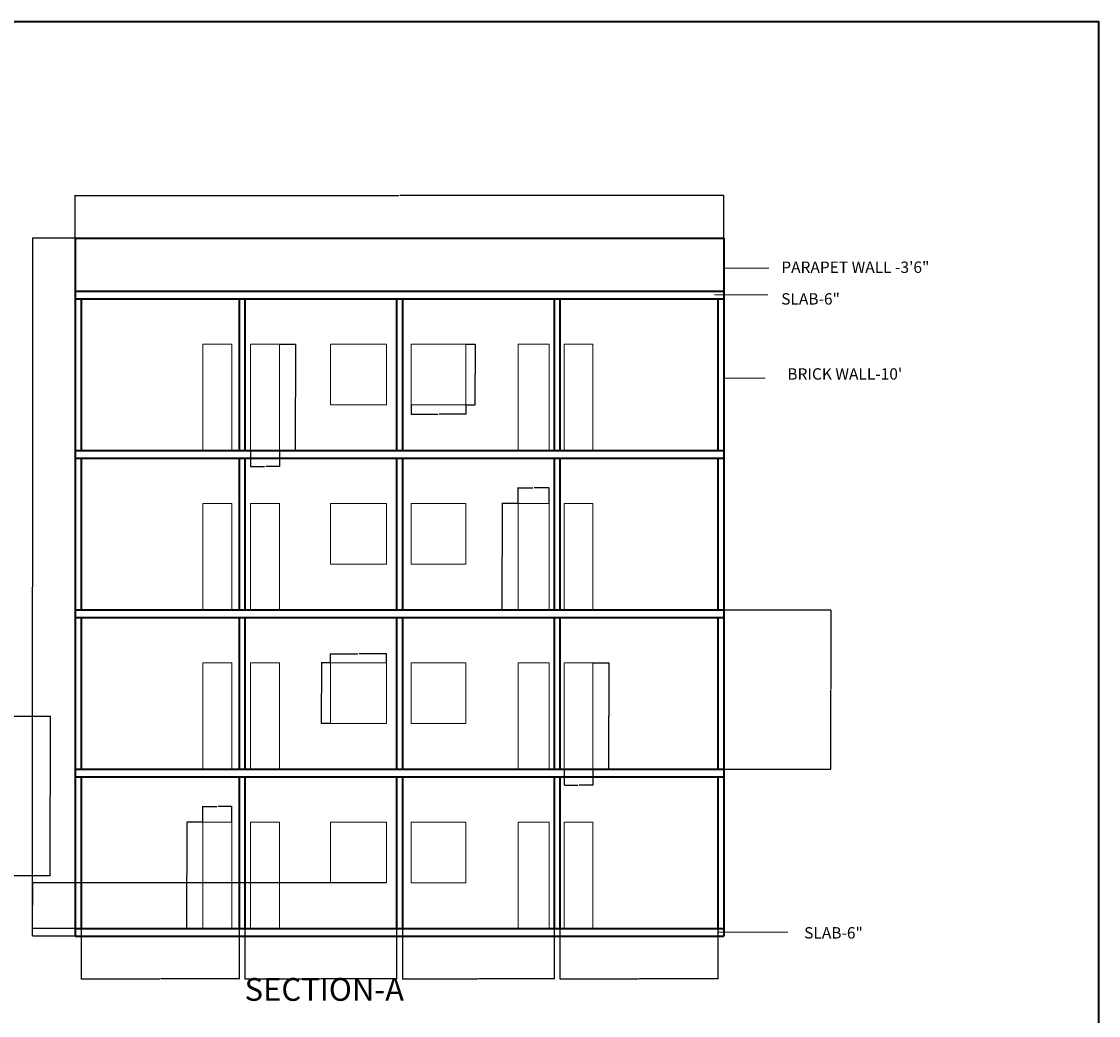
# Model space of a CAD drawing. Units: inches. Extents: x 1944 to 3454, y 1352 to 3055.
# Tile 17 of 17: x 2602 to 3454, y 2269 to 3055. Entities that reach past the tile are written whole.
import ezdxf

# ---------------------------------------------------------------- set-up
doc = ezdxf.new("R2010")
doc.units = ezdxf.units.IN
for name, color, linetype, lineweight in [('A-ANNO-DIMS', 2, 'Continuous', 18), ('A-ANNO-TEXT', 7, 'Continuous', 18), ('A-ANNO-TITL', 7, 'Continuous', 30), ('A-ANNO-TTLB', 7, 'Continuous', 35), ('A-SECT', 7, 'Continuous', 40), ('A-SECT-BYND', 8, 'Continuous', 18)]:
    doc.layers.add(name, color=color, linetype=linetype, lineweight=lineweight)
doc.styles.get("Standard").update_dxf_attribs({"font": 'arial.ttf'})
doc.dimstyles.get("Standard").update_dxf_attribs({"dimtxt": 0.18, "dimasz": 0.18, "dimexe": 0.18, "dimexo": 0.0625, "dimgap": 0.09, "dimtad": 0, "dimtih": 1, "dimtoh": 1, "dimdec": 4, "dimzin": 0, "dimdsep": 46, "dimtxsty": 'Standard', "dimcen": 0.09, "dimadec": 0, "dimazin": 0, "dimtfac": 1, "dimtdec": 4, "dimtofl": 0, "dimtmove": 0, "dimatfit": 3, "dimfxl": 1, "dimtolj": 1, "dimtzin": 0, "dimarcsym": 0})

# ---------------------------------------------------------------- blocks, each defined once
blk = doc.blocks.new('SECT-DOOR-22.85IN-01')
for p, q in [((0, 84), (0, 0)), ((0, 84), (22.85, 84)), ((22.85, 84), (22.85, 0))]:
    blk.add_line(p, q)
blk = doc.blocks.new('SECT-DOOR-23.10IN-01')
for p, q in [((0, 84), (0, 0)), ((0, 84), (23.1, 84)), ((23.1, 84), (23.1, 0))]:
    blk.add_line(p, q)
blk = doc.blocks.new('SECT-DOOR-24.49IN-01')
for p, q in [((0, 84), (0, 0)), ((0, 84), (24.49, 84)), ((24.49, 84), (24.49, 0))]:
    blk.add_line(p, q)
blk = doc.blocks.new('SECT-DOOR-22.62IN-01')
for p, q in [((0, 84), (0, 0)), ((0, 84), (22.62, 84)), ((22.62, 84), (22.62, 0))]:
    blk.add_line(p, q)
blk = doc.blocks.new('SECT-GLAZ-44.19IN-01')
for p, q in [((0, 48), (0, 0)), ((0, 48), (44.19, 48)), ((44.19, 48), (44.19, 0)), ((0, 0), (44.19, 0))]:
    blk.add_line(p, q)
blk = doc.blocks.new('SECT-GLAZ-43.38IN-01')
for p, q in [((0, 48), (0, 0)), ((0, 48), (43.38, 48)), ((43.38, 48), (43.38, 0)), ((0, 0), (43.38, 0))]:
    blk.add_line(p, q)
blk = doc.blocks.new('*D172')
at = {"layer": 'A-ANNO-DIMS', "color": 0, "lineweight": -2, "transparency": 16777216}
for p, q in [((2745.67, 2421.38), (2732.95, 2421.38)), ((2733.13, 2421.2), (2733.13, 2379.57)), ((2733.13, 2337.56), (2733.13, 2379.2)), ((2745.67, 2337.38), (2732.95, 2337.38))]:
    blk.add_line(p, q, dxfattribs=at)
at = {"layer": 'A-ANNO-DIMS', "color": 0, "transparency": 16777216}
for points in [[(2733.1, 2421.2), (2733.16, 2421.2), (2733.13, 2421.38)], [(2733.1, 2337.56), (2733.16, 2337.56), (2733.13, 2337.38)]]:
    blk.add_solid(points, dxfattribs=at)
at = {"layer": 'Defpoints', "color": 0, "transparency": 16777216}
for p in [(2733.13, 2421.38), (2745.73, 2421.38), (2745.73, 2337.38)]:
    blk.add_point(p, dxfattribs=at)
at = {"layer": 'A-ANNO-DIMS', "color": 0, "transparency": 16777216, "insert": (2733.13, 2379.38), "char_height": 0.18, "attachment_point": 5}
blk.add_mtext('\\A1;DOOR 84 TYP.', dxfattribs=at)
blk = doc.blocks.new('*D173')
at = {"layer": 'A-ANNO-DIMS', "color": 0, "lineweight": -2, "transparency": 16777216}
for p, q in [((2745.73, 2421.45), (2745.73, 2434.16)), ((2745.91, 2433.98), (2756.63, 2433.98)), ((2768.4, 2433.98), (2757.69, 2433.98)), ((2768.58, 2421.45), (2768.58, 2434.16))]:
    blk.add_line(p, q, dxfattribs=at)
at = {"layer": 'A-ANNO-DIMS', "color": 0, "transparency": 16777216}
for points in [[(2745.91, 2434.01), (2745.91, 2433.95), (2745.73, 2433.98)], [(2768.4, 2434.01), (2768.4, 2433.95), (2768.58, 2433.98)]]:
    blk.add_solid(points, dxfattribs=at)
at = {"layer": 'Defpoints', "color": 0, "transparency": 16777216}
for p in [(2768.58, 2433.98), (2745.73, 2421.38), (2768.58, 2421.38)]:
    blk.add_point(p, dxfattribs=at)
at = {"layer": 'A-ANNO-DIMS', "color": 0, "transparency": 16777216, "insert": (2757.16, 2433.98), "char_height": 0.18, "attachment_point": 5}
blk.add_mtext('\\A1;23 TYP.', dxfattribs=at)
blk = doc.blocks.new('*D174')
at = {"layer": 'A-ANNO-DIMS', "color": 0, "lineweight": -2, "transparency": 16777216}
for p, q in [((2806.45, 2799.38), (2819.17, 2799.38)), ((2818.99, 2799.2), (2818.99, 2757.57)), ((2818.99, 2715.56), (2818.99, 2757.2)), ((2806.45, 2715.38), (2819.17, 2715.38))]:
    blk.add_line(p, q, dxfattribs=at)
at = {"layer": 'A-ANNO-DIMS', "color": 0, "transparency": 16777216}
for points in [[(2818.96, 2799.2), (2819.02, 2799.2), (2818.99, 2799.38)], [(2818.96, 2715.56), (2819.02, 2715.56), (2818.99, 2715.38)]]:
    blk.add_solid(points, dxfattribs=at)
at = {"layer": 'Defpoints', "color": 0, "transparency": 16777216}
for p in [(2806.39, 2799.38), (2818.99, 2799.38), (2806.39, 2715.38)]:
    blk.add_point(p, dxfattribs=at)
at = {"layer": 'A-ANNO-DIMS', "color": 0, "transparency": 16777216, "insert": (2818.99, 2757.38), "char_height": 0.18, "attachment_point": 5}
blk.add_mtext('\\A1;DOOR 84 TYP.', dxfattribs=at)
blk = doc.blocks.new('*D175')
at = {"layer": 'A-ANNO-DIMS', "color": 0, "lineweight": -2, "transparency": 16777216}
for p, q in [((2783.29, 2715.32), (2783.29, 2702.6)), ((2806.39, 2715.32), (2806.39, 2702.6)), ((2783.47, 2702.78), (2794.31, 2702.78)), ((2806.21, 2702.78), (2795.37, 2702.78))]:
    blk.add_line(p, q, dxfattribs=at)
at = {"layer": 'A-ANNO-DIMS', "color": 0, "transparency": 16777216}
for points in [[(2783.47, 2702.81), (2783.47, 2702.75), (2783.29, 2702.78)], [(2806.21, 2702.81), (2806.21, 2702.75), (2806.39, 2702.78)]]:
    blk.add_solid(points, dxfattribs=at)
at = {"layer": 'Defpoints', "color": 0, "transparency": 16777216}
for p in [(2783.29, 2715.38), (2806.39, 2715.38), (2806.39, 2702.78)]:
    blk.add_point(p, dxfattribs=at)
at = {"layer": 'A-ANNO-DIMS', "color": 0, "transparency": 16777216, "insert": (2794.84, 2702.78), "char_height": 0.18, "attachment_point": 5}
blk.add_mtext('\\A1;23 TYP.', dxfattribs=at)
blk = doc.blocks.new('*D176')
at = {"layer": 'A-ANNO-DIMS', "color": 0, "lineweight": -2, "transparency": 16777216}
for p, q in [((2994.82, 2673.38), (2982.11, 2673.38)), ((2982.29, 2673.2), (2982.29, 2631.57)), ((2982.29, 2589.56), (2982.29, 2631.2)), ((2994.82, 2589.38), (2982.11, 2589.38))]:
    blk.add_line(p, q, dxfattribs=at)
at = {"layer": 'A-ANNO-DIMS', "color": 0, "transparency": 16777216}
for points in [[(2982.26, 2673.2), (2982.32, 2673.2), (2982.29, 2673.38)], [(2982.26, 2589.56), (2982.32, 2589.56), (2982.29, 2589.38)]]:
    blk.add_solid(points, dxfattribs=at)
at = {"layer": 'Defpoints', "color": 0, "transparency": 16777216}
for p in [(2982.29, 2673.38), (2994.89, 2673.38), (2994.89, 2589.38)]:
    blk.add_point(p, dxfattribs=at)
at = {"layer": 'A-ANNO-DIMS', "color": 0, "transparency": 16777216, "insert": (2982.29, 2631.38), "char_height": 0.18, "attachment_point": 5}
blk.add_mtext('\\A1;DOOR 84 TYP.', dxfattribs=at)
blk = doc.blocks.new('*D177')
at = {"layer": 'A-ANNO-DIMS', "color": 0, "lineweight": -2, "transparency": 16777216}
for p, q in [((2994.89, 2673.45), (2994.89, 2686.16)), ((2995.07, 2685.98), (3006.6, 2685.98)), ((3019.2, 2685.98), (3007.66, 2685.98)), ((3019.38, 2673.45), (3019.38, 2686.16))]:
    blk.add_line(p, q, dxfattribs=at)
at = {"layer": 'A-ANNO-DIMS', "color": 0, "transparency": 16777216}
for points in [[(2995.07, 2686.01), (2995.07, 2685.95), (2994.89, 2685.98)], [(3019.2, 2686.01), (3019.2, 2685.95), (3019.38, 2685.98)]]:
    blk.add_solid(points, dxfattribs=at)
at = {"layer": 'Defpoints', "color": 0, "transparency": 16777216}
for p in [(3019.38, 2685.98), (2994.89, 2673.38), (3019.38, 2673.38)]:
    blk.add_point(p, dxfattribs=at)
at = {"layer": 'A-ANNO-DIMS', "color": 0, "transparency": 16777216, "insert": (3007.13, 2685.98), "char_height": 0.18, "attachment_point": 5}
blk.add_mtext('\\A1;24 TYP.', dxfattribs=at)
blk = doc.blocks.new('*D178')
at = {"layer": 'A-ANNO-DIMS', "color": 0, "lineweight": -2, "transparency": 16777216}
for p, q in [((3054.1, 2547.38), (3066.81, 2547.38)), ((3066.63, 2547.2), (3066.63, 2505.57)), ((3066.63, 2463.56), (3066.63, 2505.2)), ((3054.1, 2463.38), (3066.81, 2463.38))]:
    blk.add_line(p, q, dxfattribs=at)
at = {"layer": 'A-ANNO-DIMS', "color": 0, "transparency": 16777216}
for points in [[(3066.6, 2547.2), (3066.66, 2547.2), (3066.63, 2547.38)], [(3066.6, 2463.56), (3066.66, 2463.56), (3066.63, 2463.38)]]:
    blk.add_solid(points, dxfattribs=at)
at = {"layer": 'Defpoints', "color": 0, "transparency": 16777216}
for p in [(3054.03, 2547.38), (3066.63, 2547.38), (3054.03, 2463.38)]:
    blk.add_point(p, dxfattribs=at)
at = {"layer": 'A-ANNO-DIMS', "color": 0, "transparency": 16777216, "insert": (3066.63, 2505.38), "char_height": 0.18, "attachment_point": 5}
blk.add_mtext('\\A1;DOOR 84 TYP.', dxfattribs=at)
blk = doc.blocks.new('*D179')
at = {"layer": 'A-ANNO-DIMS', "color": 0, "lineweight": -2, "transparency": 16777216}
for p, q in [((3031.42, 2463.32), (3031.42, 2450.6)), ((3054.03, 2463.32), (3054.03, 2450.6)), ((3031.6, 2450.78), (3042.2, 2450.78)), ((3053.85, 2450.78), (3043.26, 2450.78))]:
    blk.add_line(p, q, dxfattribs=at)
at = {"layer": 'A-ANNO-DIMS', "color": 0, "transparency": 16777216}
for points in [[(3031.6, 2450.81), (3031.6, 2450.75), (3031.42, 2450.78)], [(3053.85, 2450.81), (3053.85, 2450.75), (3054.03, 2450.78)]]:
    blk.add_solid(points, dxfattribs=at)
at = {"layer": 'Defpoints', "color": 0, "transparency": 16777216}
for p in [(3031.42, 2463.38), (3054.03, 2463.38), (3054.03, 2450.78)]:
    blk.add_point(p, dxfattribs=at)
at = {"layer": 'A-ANNO-DIMS', "color": 0, "transparency": 16777216, "insert": (3042.73, 2450.78), "char_height": 0.18, "attachment_point": 5}
blk.add_mtext('\\A1;23 TYP.', dxfattribs=at)
blk = doc.blocks.new('*D180')
at = {"layer": 'A-ANNO-DIMS', "color": 0, "lineweight": -2, "transparency": 16777216}
for p, q in [((2846.48, 2547.38), (2839.17, 2547.38)), ((2839.35, 2547.2), (2839.35, 2523.57)), ((2839.35, 2499.56), (2839.35, 2523.2)), ((2846.48, 2499.38), (2839.17, 2499.38))]:
    blk.add_line(p, q, dxfattribs=at)
at = {"layer": 'A-ANNO-DIMS', "color": 0, "transparency": 16777216}
for points in [[(2839.32, 2547.2), (2839.38, 2547.2), (2839.35, 2547.38)], [(2839.32, 2499.56), (2839.38, 2499.56), (2839.35, 2499.38)]]:
    blk.add_solid(points, dxfattribs=at)
at = {"layer": 'Defpoints', "color": 0, "transparency": 16777216}
for p in [(2839.35, 2547.38), (2846.55, 2547.38), (2846.55, 2499.38)]:
    blk.add_point(p, dxfattribs=at)
at = {"layer": 'A-ANNO-DIMS', "color": 0, "transparency": 16777216, "insert": (2839.35, 2523.38), "char_height": 0.18, "attachment_point": 5}
blk.add_mtext('\\A1;GLAZING 48 TYP.', dxfattribs=at)
blk = doc.blocks.new('*D181')
at = {"layer": 'A-ANNO-DIMS', "color": 0, "lineweight": -2, "transparency": 16777216}
for p, q in [((2846.55, 2547.45), (2846.55, 2554.76)), ((2846.73, 2554.58), (2868.11, 2554.58)), ((2890.56, 2554.58), (2869.17, 2554.58)), ((2890.74, 2547.45), (2890.74, 2554.76))]:
    blk.add_line(p, q, dxfattribs=at)
at = {"layer": 'A-ANNO-DIMS', "color": 0, "transparency": 16777216}
for points in [[(2846.73, 2554.61), (2846.73, 2554.55), (2846.55, 2554.58)], [(2890.56, 2554.61), (2890.56, 2554.55), (2890.74, 2554.58)]]:
    blk.add_solid(points, dxfattribs=at)
at = {"layer": 'Defpoints', "color": 0, "transparency": 16777216}
for p in [(2890.74, 2554.58), (2846.55, 2547.38), (2890.74, 2547.38)]:
    blk.add_point(p, dxfattribs=at)
at = {"layer": 'A-ANNO-DIMS', "color": 0, "transparency": 16777216, "insert": (2868.64, 2554.58), "char_height": 0.18, "attachment_point": 5}
blk.add_mtext('\\A1;44 TYP.', dxfattribs=at)
blk = doc.blocks.new('*D182')
at = {"layer": 'A-ANNO-DIMS', "color": 0, "lineweight": -2, "transparency": 16777216}
for p, q in [((2953.72, 2799.38), (2961.03, 2799.38)), ((2960.85, 2799.2), (2960.85, 2775.57)), ((2960.85, 2751.56), (2960.85, 2775.2)), ((2953.72, 2751.38), (2961.03, 2751.38))]:
    blk.add_line(p, q, dxfattribs=at)
at = {"layer": 'A-ANNO-DIMS', "color": 0, "transparency": 16777216}
for points in [[(2960.82, 2799.2), (2960.88, 2799.2), (2960.85, 2799.38)], [(2960.82, 2751.56), (2960.88, 2751.56), (2960.85, 2751.38)]]:
    blk.add_solid(points, dxfattribs=at)
at = {"layer": 'Defpoints', "color": 0, "transparency": 16777216}
for p in [(2953.65, 2799.38), (2960.85, 2799.38), (2953.65, 2751.38)]:
    blk.add_point(p, dxfattribs=at)
at = {"layer": 'A-ANNO-DIMS', "color": 0, "transparency": 16777216, "insert": (2960.85, 2775.38), "char_height": 0.18, "attachment_point": 5}
blk.add_mtext('\\A1;GLAZING 48 TYP.', dxfattribs=at)
blk = doc.blocks.new('*D183')
at = {"layer": 'A-ANNO-DIMS', "color": 0, "lineweight": -2, "transparency": 16777216}
for p, q in [((2910.28, 2751.32), (2910.28, 2744)), ((2953.65, 2751.32), (2953.65, 2744)), ((2910.46, 2744.18), (2931.43, 2744.18)), ((2953.47, 2744.18), (2932.5, 2744.18))]:
    blk.add_line(p, q, dxfattribs=at)
at = {"layer": 'A-ANNO-DIMS', "color": 0, "transparency": 16777216}
for points in [[(2910.46, 2744.21), (2910.46, 2744.15), (2910.28, 2744.18)], [(2953.47, 2744.21), (2953.47, 2744.15), (2953.65, 2744.18)]]:
    blk.add_solid(points, dxfattribs=at)
at = {"layer": 'Defpoints', "color": 0, "transparency": 16777216}
for p in [(2910.28, 2751.38), (2953.65, 2751.38), (2953.65, 2744.18)]:
    blk.add_point(p, dxfattribs=at)
at = {"layer": 'A-ANNO-DIMS', "color": 0, "transparency": 16777216, "insert": (2931.96, 2744.18), "char_height": 0.18, "attachment_point": 5}
blk.add_mtext('\\A1;43 TYP.', dxfattribs=at)
blk = doc.blocks.new('*D201')
at = {"layer": 'A-ANNO-DIMS', "color": 0, "lineweight": -2, "transparency": 16777216}
for p, q in [((2593.88, 2505.38), (2625.2, 2505.38)), ((2625.02, 2505.2), (2625.02, 2442.57)), ((2625.02, 2379.56), (2625.02, 2442.2)), ((2593.88, 2379.38), (2625.2, 2379.38))]:
    blk.add_line(p, q, dxfattribs=at)
at = {"layer": 'A-ANNO-DIMS', "color": 0, "transparency": 16777216}
for points in [[(2624.99, 2505.2), (2625.05, 2505.2), (2625.02, 2505.38)], [(2624.99, 2379.56), (2625.05, 2379.56), (2625.02, 2379.38)]]:
    blk.add_solid(points, dxfattribs=at)
at = {"layer": 'Defpoints', "color": 0, "transparency": 16777216}
for p in [(2593.82, 2505.38), (2625.02, 2505.38), (2593.82, 2379.38)]:
    blk.add_point(p, dxfattribs=at)
at = {"layer": 'A-ANNO-DIMS', "color": 0, "transparency": 16777216, "insert": (2625.02, 2442.38), "char_height": 0.18, "attachment_point": 5}
blk.add_mtext('\\A1;126', dxfattribs=at)
blk = doc.blocks.new('*D209')
at = {"layer": 'A-ANNO-DIMS', "color": 0, "lineweight": -2, "transparency": 16777216}
for p, q in [((2644.88, 2883.45), (2644.88, 2917.33)), ((2645.06, 2917.15), (2900.73, 2917.15)), ((3157.2, 2917.15), (2901.52, 2917.15)), ((3157.38, 2883.45), (3157.38, 2917.33))]:
    blk.add_line(p, q, dxfattribs=at)
at = {"layer": 'A-ANNO-DIMS', "color": 0, "transparency": 16777216}
for points in [[(2645.06, 2917.18), (2645.06, 2917.12), (2644.88, 2917.15)], [(3157.2, 2917.18), (3157.2, 2917.12), (3157.38, 2917.15)]]:
    blk.add_solid(points, dxfattribs=at)
at = {"layer": 'Defpoints', "color": 0, "transparency": 16777216}
for p in [(3157.38, 2917.15), (2644.88, 2883.38), (3157.38, 2883.38)]:
    blk.add_point(p, dxfattribs=at)
at = {"layer": 'A-ANNO-DIMS', "color": 0, "transparency": 16777216, "insert": (2901.13, 2917.15), "char_height": 0.18, "attachment_point": 5}
blk.add_mtext('\\A1;512.5', dxfattribs=at)
blk = doc.blocks.new('*D210')
at = {"layer": 'A-ANNO-DIMS', "color": 0, "lineweight": -2, "transparency": 16777216}
for p, q in [((2644.81, 2883.38), (2610.93, 2883.38)), ((2611.11, 2883.2), (2611.11, 2607.57)), ((2611.11, 2331.56), (2611.11, 2607.2)), ((2644.81, 2331.38), (2610.93, 2331.38))]:
    blk.add_line(p, q, dxfattribs=at)
at = {"layer": 'A-ANNO-DIMS', "color": 0, "transparency": 16777216}
for points in [[(2611.08, 2883.2), (2611.14, 2883.2), (2611.11, 2883.38)], [(2611.08, 2331.56), (2611.14, 2331.56), (2611.11, 2331.38)]]:
    blk.add_solid(points, dxfattribs=at)
at = {"layer": 'Defpoints', "color": 0, "transparency": 16777216}
for p in [(2611.11, 2883.38), (2644.88, 2883.38), (2644.88, 2331.38)]:
    blk.add_point(p, dxfattribs=at)
at = {"layer": 'A-ANNO-DIMS', "color": 0, "transparency": 16777216, "insert": (2611.11, 2607.38), "char_height": 0.18, "attachment_point": 5}
blk.add_mtext('\\A1;552', dxfattribs=at)
blk = doc.blocks.new('*D211')
at = {"layer": 'A-ANNO-DIMS', "color": 0, "lineweight": -2, "transparency": 16777216}
for p, q in [((3157.44, 2589.38), (3242.15, 2589.38)), ((3241.97, 2589.2), (3241.97, 2526.57)), ((3241.97, 2463.56), (3241.97, 2526.2)), ((3157.44, 2463.38), (3242.15, 2463.38))]:
    blk.add_line(p, q, dxfattribs=at)
at = {"layer": 'A-ANNO-DIMS', "color": 0, "transparency": 16777216}
for points in [[(3241.94, 2589.2), (3242, 2589.2), (3241.97, 2589.38)], [(3241.94, 2463.56), (3242, 2463.56), (3241.97, 2463.38)]]:
    blk.add_solid(points, dxfattribs=at)
at = {"layer": 'Defpoints', "color": 0, "transparency": 16777216}
for p in [(3157.38, 2589.38), (3241.97, 2589.38), (3157.38, 2463.38)]:
    blk.add_point(p, dxfattribs=at)
at = {"layer": 'A-ANNO-DIMS', "color": 0, "transparency": 16777216, "insert": (3241.97, 2526.38), "char_height": 0.18, "attachment_point": 5}
blk.add_mtext('\\A1;126', dxfattribs=at)
blk = doc.blocks.new('*D212')
at = {"layer": 'A-ANNO-DIMS', "color": 0, "lineweight": -2, "transparency": 16777216}
for p, q in [((2649.38, 2337.32), (2649.38, 2297.43)), ((2774.38, 2337.32), (2774.38, 2297.43)), ((2649.56, 2297.61), (2711.59, 2297.61)), ((2774.2, 2297.61), (2712.16, 2297.61))]:
    blk.add_line(p, q, dxfattribs=at)
at = {"layer": 'A-ANNO-DIMS', "color": 0, "transparency": 16777216}
for points in [[(2649.56, 2297.64), (2649.56, 2297.58), (2649.38, 2297.61)], [(2774.2, 2297.64), (2774.2, 2297.58), (2774.38, 2297.61)]]:
    blk.add_solid(points, dxfattribs=at)
at = {"layer": 'Defpoints', "color": 0, "transparency": 16777216}
for p in [(2649.38, 2337.38), (2774.38, 2337.38), (2774.38, 2297.61)]:
    blk.add_point(p, dxfattribs=at)
at = {"layer": 'A-ANNO-DIMS', "color": 0, "transparency": 16777216, "insert": (2711.88, 2297.61), "char_height": 0.18, "attachment_point": 5}
blk.add_mtext('\\A1;125', dxfattribs=at)
blk = doc.blocks.new('*D213')
at = {"layer": 'A-ANNO-DIMS', "color": 0, "lineweight": -2, "transparency": 16777216}
for p, q in [((2778.88, 2337.32), (2778.88, 2297.43)), ((2898.88, 2337.32), (2898.88, 2297.43)), ((2779.06, 2297.61), (2838.6, 2297.61)), ((2898.7, 2297.61), (2839.16, 2297.61))]:
    blk.add_line(p, q, dxfattribs=at)
at = {"layer": 'A-ANNO-DIMS', "color": 0, "transparency": 16777216}
for points in [[(2779.06, 2297.64), (2779.06, 2297.58), (2778.88, 2297.61)], [(2898.7, 2297.64), (2898.7, 2297.58), (2898.88, 2297.61)]]:
    blk.add_solid(points, dxfattribs=at)
at = {"layer": 'Defpoints', "color": 0, "transparency": 16777216}
for p in [(2778.88, 2337.38), (2898.88, 2337.38), (2898.88, 2297.61)]:
    blk.add_point(p, dxfattribs=at)
at = {"layer": 'A-ANNO-DIMS', "color": 0, "transparency": 16777216, "insert": (2838.88, 2297.61), "char_height": 0.18, "attachment_point": 5}
blk.add_mtext('\\A1;120', dxfattribs=at)
blk = doc.blocks.new('*D214')
at = {"layer": 'A-ANNO-DIMS', "color": 0, "lineweight": -2, "transparency": 16777216}
for p, q in [((2903.38, 2337.32), (2903.38, 2297.43)), ((3023.38, 2337.32), (3023.38, 2297.43)), ((2903.56, 2297.61), (2963.1, 2297.61)), ((3023.2, 2297.61), (2963.66, 2297.61))]:
    blk.add_line(p, q, dxfattribs=at)
at = {"layer": 'A-ANNO-DIMS', "color": 0, "transparency": 16777216}
for points in [[(2903.56, 2297.64), (2903.56, 2297.58), (2903.38, 2297.61)], [(3023.2, 2297.64), (3023.2, 2297.58), (3023.38, 2297.61)]]:
    blk.add_solid(points, dxfattribs=at)
at = {"layer": 'Defpoints', "color": 0, "transparency": 16777216}
for p in [(2903.38, 2337.38), (3023.38, 2337.38), (3023.38, 2297.61)]:
    blk.add_point(p, dxfattribs=at)
at = {"layer": 'A-ANNO-DIMS', "color": 0, "transparency": 16777216, "insert": (2963.38, 2297.61), "char_height": 0.18, "attachment_point": 5}
blk.add_mtext('\\A1;120', dxfattribs=at)
blk = doc.blocks.new('*D215')
at = {"layer": 'A-ANNO-DIMS', "color": 0, "lineweight": -2, "transparency": 16777216}
for p, q in [((3027.88, 2337.32), (3027.88, 2297.43)), ((3152.88, 2337.32), (3152.88, 2297.43)), ((3028.06, 2297.61), (3090.09, 2297.61)), ((3152.7, 2297.61), (3090.66, 2297.61))]:
    blk.add_line(p, q, dxfattribs=at)
at = {"layer": 'A-ANNO-DIMS', "color": 0, "transparency": 16777216}
for points in [[(3028.06, 2297.64), (3028.06, 2297.58), (3027.88, 2297.61)], [(3152.7, 2297.64), (3152.7, 2297.58), (3152.88, 2297.61)]]:
    blk.add_solid(points, dxfattribs=at)
at = {"layer": 'Defpoints', "color": 0, "transparency": 16777216}
for p in [(3027.88, 2337.38), (3152.88, 2337.38), (3152.88, 2297.61)]:
    blk.add_point(p, dxfattribs=at)
at = {"layer": 'A-ANNO-DIMS', "color": 0, "transparency": 16777216, "insert": (3090.38, 2297.61), "char_height": 0.18, "attachment_point": 5}
blk.add_mtext('\\A1;125', dxfattribs=at)
blk = doc.blocks.new('*D216')
at = {"layer": 'A-ANNO-DIMS', "color": 0, "lineweight": -2, "transparency": 16777216}
for p, q in [((2890.68, 2373.38), (2610.93, 2373.38)), ((2611.11, 2373.2), (2611.11, 2355.57)), ((2611.11, 2337.56), (2611.11, 2355.2)), ((2898.81, 2337.38), (2610.93, 2337.38))]:
    blk.add_line(p, q, dxfattribs=at)
at = {"layer": 'A-ANNO-DIMS', "color": 0, "transparency": 16777216}
for points in [[(2611.08, 2373.2), (2611.14, 2373.2), (2611.11, 2373.38)], [(2611.08, 2337.56), (2611.14, 2337.56), (2611.11, 2337.38)]]:
    blk.add_solid(points, dxfattribs=at)
at = {"layer": 'Defpoints', "color": 0, "transparency": 16777216}
for p in [(2611.11, 2373.38), (2890.74, 2373.38), (2898.88, 2337.38)]:
    blk.add_point(p, dxfattribs=at)
at = {"layer": 'A-ANNO-DIMS', "color": 0, "transparency": 16777216, "insert": (2611.11, 2355.38), "char_height": 0.18, "attachment_point": 5}
blk.add_mtext('\\A1;36', dxfattribs=at)

msp = doc.modelspace()

# ---------------------------------------------------------------- linework, layer by layer
at = {"layer": 'A-ANNO-TEXT'}
for p, q in [((3157.375, 2859.621), (3193.12, 2859.621)), ((3150.241, 2838.525), (3192.374, 2838.525)), ((3157.375, 2772.453), (3190.268, 2772.453)), ((3153.018, 2334.491), (3208.197, 2334.491))]:
    msp.add_line(p, q, dxfattribs=at)
at = {"layer": 'A-ANNO-TTLB'}
msp.add_lwpolyline([(1943.914, 3054.605), (3453.633, 3054.605), (3453.633, 1351.76), (1943.914, 1351.76)], close=True, dxfattribs=at)
at = {"layer": 'A-SECT'}
for p, q in [((2644.875, 2883.384), (2644.875, 2709.384)), ((2644.875, 2883.384), (3157.375, 2883.384)), ((3157.375, 2883.384), (3157.375, 2709.384)), ((2644.875, 2841.384), (3157.375, 2841.384)), ((2644.875, 2835.384), (3157.375, 2835.384)), ((2649.375, 2835.384), (2649.375, 2715.384)), ((2774.375, 2835.384), (2774.375, 2715.384)), ((2778.875, 2835.384), (2778.875, 2715.384)), ((2778.875, 2835.384), (2778.875, 2715.384)), ((2898.875, 2835.384), (2898.875, 2715.384)), ((2903.375, 2835.384), (2903.375, 2715.384)), ((3023.375, 2835.384), (3023.375, 2715.384)), ((3027.875, 2835.384), (3027.875, 2715.384)), ((3152.875, 2835.384), (3152.875, 2715.384)), ((2644.875, 2757.384), (2644.875, 2583.384)), ((3157.375, 2757.384), (3157.375, 2583.384)), ((2644.875, 2715.384), (3157.375, 2715.384)), ((2644.875, 2709.384), (3157.375, 2709.384)), ((2649.375, 2709.384), (2649.375, 2589.384)), ((2774.375, 2709.384), (2774.375, 2589.384)), ((2778.875, 2709.384), (2778.875, 2589.384)), ((2778.875, 2709.384), (2778.875, 2589.384)), ((2898.875, 2709.384), (2898.875, 2589.384)), ((2903.375, 2709.384), (2903.375, 2589.384)), ((3023.375, 2709.384), (3023.375, 2589.384)), ((3027.875, 2709.384), (3027.875, 2589.384)), ((3152.875, 2709.384), (3152.875, 2589.384)), ((2644.875, 2631.384), (2644.875, 2457.384)), ((3157.375, 2631.384), (3157.375, 2457.384)), ((2644.875, 2589.384), (3157.375, 2589.384)), ((2644.875, 2583.384), (3157.375, 2583.384)), ((2649.375, 2583.384), (2649.375, 2463.384)), ((2774.375, 2583.384), (2774.375, 2463.384)), ((2778.875, 2583.384), (2778.875, 2463.384)), ((2778.875, 2583.384), (2778.875, 2463.384)), ((2898.875, 2583.384), (2898.875, 2463.384)), ((2903.375, 2583.384), (2903.375, 2463.384)), ((3023.375, 2583.384), (3023.375, 2463.384)), ((3027.875, 2583.384), (3027.875, 2463.384)), ((3152.875, 2583.384), (3152.875, 2463.384)), ((2644.875, 2505.384), (2644.875, 2331.384)), ((3157.375, 2505.384), (3157.375, 2331.384)), ((2644.875, 2463.384), (3157.375, 2463.384)), ((2644.875, 2457.384), (3157.375, 2457.384)), ((2649.375, 2457.384), (2649.375, 2337.384)), ((2774.375, 2457.384), (2774.375, 2337.384)), ((2778.875, 2457.384), (2778.875, 2337.384)), ((2778.875, 2457.384), (2778.875, 2337.384)), ((2898.875, 2457.384), (2898.875, 2337.384)), ((2903.375, 2457.384), (2903.375, 2337.384)), ((3023.375, 2457.384), (3023.375, 2337.384)), ((3027.875, 2457.384), (3027.875, 2337.384)), ((3152.875, 2457.384), (3152.875, 2337.384)), ((2644.875, 2337.384), (3157.375, 2337.384)), ((2644.875, 2331.384), (3157.375, 2331.384))]:
    msp.add_line(p, q, dxfattribs=at)

# ---------------------------------------------------------------- block references
at = {"layer": 'A-SECT-BYND'}
for name, p in [('SECT-DOOR-22.85IN-01', (2745.734, 2715.384)), ('SECT-DOOR-23.10IN-01', (2783.292, 2715.384)), ('SECT-GLAZ-44.19IN-01', (2846.547, 2751.384)), ('SECT-GLAZ-43.38IN-01', (2910.276, 2751.384)), ('SECT-DOOR-24.49IN-01', (2994.887, 2715.384)), ('SECT-DOOR-22.62IN-01', (3031.419, 2715.384)), ('SECT-DOOR-22.85IN-01', (2745.734, 2589.384)), ('SECT-DOOR-23.10IN-01', (2783.292, 2589.384)), ('SECT-GLAZ-44.19IN-01', (2846.547, 2625.384)), ('SECT-GLAZ-43.38IN-01', (2910.276, 2625.384)), ('SECT-DOOR-24.49IN-01', (2994.887, 2589.384)), ('SECT-DOOR-22.62IN-01', (3031.419, 2589.384)), ('SECT-DOOR-22.85IN-01', (2745.734, 2463.384)), ('SECT-DOOR-23.10IN-01', (2783.292, 2463.384)), ('SECT-GLAZ-44.19IN-01', (2846.547, 2499.384)), ('SECT-GLAZ-43.38IN-01', (2910.276, 2499.384)), ('SECT-DOOR-24.49IN-01', (2994.887, 2463.384)), ('SECT-DOOR-22.62IN-01', (3031.419, 2463.384)), ('SECT-DOOR-22.85IN-01', (2745.734, 2337.384)), ('SECT-DOOR-23.10IN-01', (2783.292, 2337.384)), ('SECT-GLAZ-44.19IN-01', (2846.547, 2373.384)), ('SECT-GLAZ-43.38IN-01', (2910.276, 2373.384)), ('SECT-DOOR-24.49IN-01', (2994.887, 2337.384)), ('SECT-DOOR-22.62IN-01', (3031.419, 2337.384))]:
    msp.add_blockref(name, p, dxfattribs=at)

# ---------------------------------------------------------------- texts
at = {"layer": 'A-ANNO-TEXT', "char_height": 9, "attachment_point": 1}
for s, width, insert in [('PARAPET WALL -3\'6"', 316.15499, (3202.92, 2864.819)), ('SLAB-6"', 56.98345, (3202.868, 2839.758)), ("BRICK WALL-10'", 266.71804, (3207.688, 2780.4)), ('SLAB-6"', 288.06232, (3220.995, 2338.443))]:
    msp.add_mtext_dynamic_manual_height_columns(s, width=width, gutter_width=12.5, heights=[0], dxfattribs=dict(at, insert=insert))
at = {"layer": 'A-ANNO-TITL', "insert": (2778.623, 2298.207), "char_height": 18, "attachment_point": 1}
msp.add_mtext_dynamic_manual_height_columns('SECTION-A', width=334.27577, gutter_width=12.5, heights=[0], dxfattribs=at)

# ---------------------------------------------------------------- dimensions: what is measured, and where the dimension line sits
at = {"layer": 'A-ANNO-DIMS'}
for base, p1, p2, override, picture, middle in [((3157.375, 2917.154), (2644.875, 2883.384), (3157.375, 2883.384), {"dimdec": 1, "dimlfac": 1, "dimrnd": 0, "dimzin": 0, "dimdsep": 46, "dimlunit": 2}, '*D209', (2901.125, 2917.154)), ((2774.375, 2297.614), (2649.375, 2337.384), (2774.375, 2337.384), {"dimdec": 0, "dimlfac": 1, "dimrnd": 0, "dimzin": 0, "dimdsep": 46, "dimlunit": 2}, '*D212', (2711.875, 2297.614)), ((2898.875, 2297.614), (2778.875, 2337.384), (2898.875, 2337.384), {"dimdec": 0, "dimlfac": 1, "dimrnd": 0, "dimzin": 0, "dimdsep": 46, "dimlunit": 2}, '*D213', (2838.875, 2297.614)), ((3023.375, 2297.614), (2903.375, 2337.384), (3023.375, 2337.384), {"dimdec": 0, "dimlfac": 1, "dimrnd": 0, "dimzin": 0, "dimdsep": 46, "dimlunit": 2}, '*D214', (2963.375, 2297.614)), ((3152.875, 2297.614), (3027.875, 2337.384), (3152.875, 2337.384), {"dimdec": 0, "dimlfac": 1, "dimrnd": 0, "dimzin": 0, "dimdsep": 46, "dimlunit": 2}, '*D215', (3090.375, 2297.614))]:
    dim = msp.add_linear_dim(base=base, p1=p1, p2=p2, dimstyle='Standard', override=override, dxfattribs=at)
    dim.commit()
    dim.dimension.update_dxf_attribs({"geometry": picture, "text_midpoint": middle})
for base, p1, p2, picture, middle in [((2611.105, 2883.384), (2644.875, 2331.384), (2644.875, 2883.384), '*D210', (2611.105, 2607.384)), ((3241.967, 2589.384), (3157.375, 2463.384), (3157.375, 2589.384), '*D211', (3241.967, 2526.384)), ((2625.022, 2505.384), (2593.822, 2379.384), (2593.822, 2505.384), '*D201', (2625.022, 2442.384)), ((2611.105, 2373.384), (2898.875, 2337.384), (2890.74, 2373.384), '*D216', (2611.105, 2355.384))]:
    dim = msp.add_linear_dim(base=base, p1=p1, p2=p2, angle=90, dimstyle='Standard', override={"dimdec": 0, "dimlfac": 1, "dimrnd": 0, "dimzin": 0, "dimdsep": 46, "dimlunit": 2}, dxfattribs=at)
    dim.commit()
    dim.dimension.update_dxf_attribs({"geometry": picture, "text_midpoint": middle})
for base, p1, p2, text, picture, middle in [((2818.991, 2799.384), (2806.391, 2715.384), (2806.391, 2799.384), 'DOOR <> TYP.', '*D174', (2818.991, 2757.384)), ((2960.853, 2799.384), (2953.653, 2751.384), (2953.653, 2799.384), 'GLAZING <> TYP.', '*D182', (2960.853, 2775.384)), ((2982.287, 2673.384), (2994.887, 2589.384), (2994.887, 2673.384), 'DOOR <> TYP.', '*D176', (2982.287, 2631.384)), ((2839.347, 2547.384), (2846.547, 2499.384), (2846.547, 2547.384), 'GLAZING <> TYP.', '*D180', (2839.347, 2523.384)), ((3066.634, 2547.384), (3054.034, 2463.384), (3054.034, 2547.384), 'DOOR <> TYP.', '*D178', (3066.634, 2505.384)), ((2733.134, 2421.384), (2745.734, 2337.384), (2745.734, 2421.384), 'DOOR <> TYP.', '*D172', (2733.134, 2379.384))]:
    dim = msp.add_linear_dim(base=base, p1=p1, p2=p2, angle=90, text=text, dimstyle='Standard', override={"dimdec": 0, "dimlfac": 1, "dimrnd": 0, "dimzin": 0, "dimdsep": 46, "dimlunit": 2}, dxfattribs=at)
    dim.commit()
    dim.dimension.update_dxf_attribs({"geometry": picture, "text_midpoint": middle})
for base, p1, p2, picture, middle in [((2953.653, 2744.184), (2910.276, 2751.384), (2953.653, 2751.384), '*D183', (2931.964, 2744.184)), ((2806.391, 2702.784), (2783.292, 2715.384), (2806.391, 2715.384), '*D175', (2794.842, 2702.784)), ((3019.381, 2685.984), (2994.887, 2673.384), (3019.381, 2673.384), '*D177', (3007.134, 2685.984)), ((2890.74, 2554.584), (2846.547, 2547.384), (2890.74, 2547.384), '*D181', (2868.643, 2554.584)), ((3054.034, 2450.784), (3031.419, 2463.384), (3054.034, 2463.384), '*D179', (3042.727, 2450.784)), ((2768.579, 2433.984), (2745.734, 2421.384), (2768.579, 2421.384), '*D173', (2757.157, 2433.984))]:
    dim = msp.add_linear_dim(base=base, p1=p1, p2=p2, text='<> TYP.', dimstyle='Standard', override={"dimdec": 0, "dimlfac": 1, "dimrnd": 0, "dimzin": 0, "dimdsep": 46, "dimlunit": 2}, dxfattribs=at)
    dim.commit()
    dim.dimension.update_dxf_attribs({"geometry": picture, "text_midpoint": middle})

doc.saveas('drawing.dxf')
